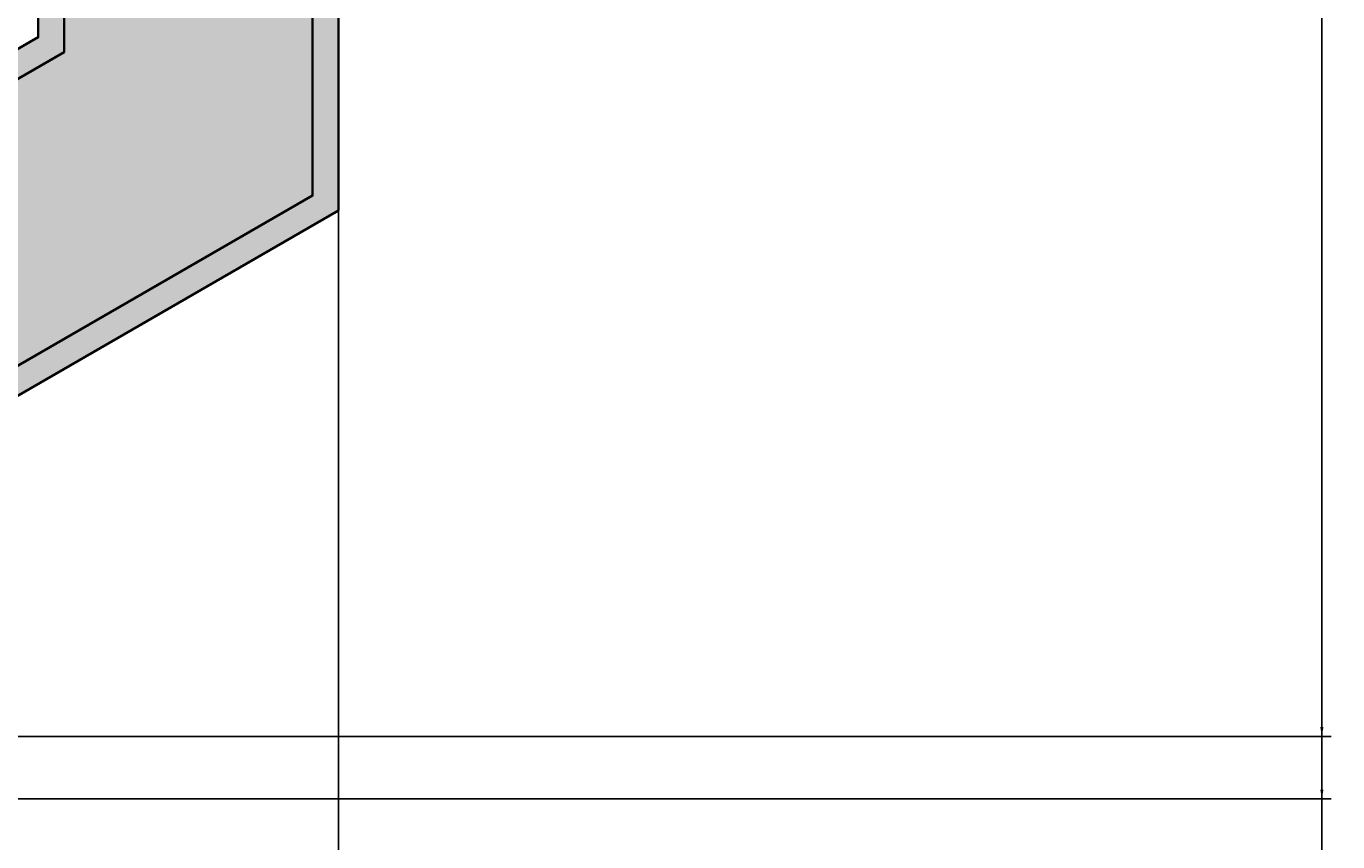
# Model space of a CAD drawing. Units: inches. Extents: x -1 to 292, y -3 to 199.
# Tile 48 of 52: x 267 to 292, y 43 to 58. Entities that reach past the tile are written whole.
import ezdxf

# ---------------------------------------------------------------- set-up
doc = ezdxf.new("R2010")
doc.units = ezdxf.units.IN
doc.header["$MEASUREMENT"] = 0
for name, color, linetype, lineweight in [('M-DIMS', 2, 'Continuous', 18), ('M-EQPM', 7, 'Continuous', 35), ('M-PATT', 8, 'Continuous', 13)]:
    doc.layers.add(name, color=color, linetype=linetype, lineweight=lineweight)
doc.styles.get("Standard").update_dxf_attribs({"font": 'arial.ttf'})
doc.dimstyles.get("Standard").update_dxf_attribs({"dimtxt": 0.18, "dimasz": 0.18, "dimexe": 0.18, "dimexo": 0.0625, "dimgap": 0.09, "dimtad": 0, "dimtih": 1, "dimtoh": 1, "dimdec": 4, "dimzin": 0, "dimdsep": 46, "dimtxsty": 'Standard', "dimcen": 0.09, "dimadec": 0, "dimazin": 0, "dimtfac": 1, "dimtdec": 4, "dimtofl": 0, "dimtmove": 0, "dimatfit": 3, "dimfxl": 1, "dimtolj": 1, "dimtzin": 0, "dimarcsym": 0})

# ---------------------------------------------------------------- blocks, each defined once
blk = doc.blocks.new('*D10')
at = {"layer": 'Defpoints', "color": 0, "transparency": 16777216}
for p in [(169.176, 99.774), (169.176, 43.391), (292.04, 43.391)]:
    blk.add_point(p, dxfattribs=at)
at = {"layer": 'M-DIMS', "color": 0, "lineweight": -2, "transparency": 16777216}
for p, q in [((169.239, 99.774), (292.22, 99.774)), ((292.04, 99.594), (292.04, 71.764)), ((292.04, 43.571), (292.04, 71.4)), ((169.239, 43.391), (292.22, 43.391))]:
    blk.add_line(p, q, dxfattribs=at)
at = {"layer": 'M-DIMS', "color": 0, "transparency": 16777216}
for points in [[(292.01, 99.594), (292.07, 99.594), (292.04, 99.774)], [(292.01, 43.571), (292.07, 43.571), (292.04, 43.391)]]:
    blk.add_solid(points, dxfattribs=at)
at = {"layer": 'M-DIMS', "color": 0, "transparency": 16777216, "insert": (292.04, 71.582), "char_height": 0.18, "attachment_point": 5}
blk.add_mtext('\\A1;56.38', dxfattribs=at)
blk = doc.blocks.new('*D25')
at = {"layer": 'Defpoints', "color": 0, "transparency": 16777216}
for p in [(273.066, 88.419), (215.241, 88.13), (273.066, -2.71)]:
    blk.add_point(p, dxfattribs=at)
at = {"layer": 'M-DIMS', "color": 0, "lineweight": -2, "transparency": 16777216}
for p, q in [((273.066, 88.357), (273.066, -2.89)), ((215.241, 88.068), (215.241, -2.89)), ((215.421, -2.71), (243.76, -2.71)), ((272.886, -2.71), (244.547, -2.71))]:
    blk.add_line(p, q, dxfattribs=at)
at = {"layer": 'M-DIMS', "color": 0, "transparency": 16777216}
for points in [[(215.421, -2.68), (215.421, -2.74), (215.241, -2.71)], [(272.886, -2.68), (272.886, -2.74), (273.066, -2.71)]]:
    blk.add_solid(points, dxfattribs=at)
at = {"layer": 'M-DIMS', "color": 0, "transparency": 16777216, "insert": (244.153, -2.71), "char_height": 0.18, "attachment_point": 5}
blk.add_mtext('\\A1;57.83', dxfattribs=at)
blk = doc.blocks.new('*D29')
at = {"layer": 'Defpoints', "color": 0, "transparency": 16777216}
for p in [(243.903, 98.567), (243.903, 44.598), (292.04, 44.598)]:
    blk.add_point(p, dxfattribs=at)
at = {"layer": 'M-DIMS', "color": 0, "lineweight": -2, "transparency": 16777216}
for p, q in [((243.966, 98.567), (292.22, 98.567)), ((292.04, 98.387), (292.04, 71.764)), ((292.04, 44.778), (292.04, 71.4)), ((243.966, 44.598), (292.22, 44.598))]:
    blk.add_line(p, q, dxfattribs=at)
at = {"layer": 'M-DIMS', "color": 0, "transparency": 16777216}
for points in [[(292.01, 98.387), (292.07, 98.387), (292.04, 98.567)], [(292.01, 44.778), (292.07, 44.778), (292.04, 44.598)]]:
    blk.add_solid(points, dxfattribs=at)
at = {"layer": 'M-DIMS', "color": 0, "transparency": 16777216, "insert": (292.04, 71.582), "char_height": 0.18, "attachment_point": 5}
blk.add_mtext('\\A1;53.97', dxfattribs=at)
blk = doc.blocks.new('*D33')
at = {"layer": 'Defpoints', "color": 0, "transparency": 16777216}
for p in [(242.955, 125.727), (292.04, 125.727), (237.933, 30.73)]:
    blk.add_point(p, dxfattribs=at)
at = {"layer": 'M-DIMS', "color": 0, "lineweight": -2, "transparency": 16777216}
for p, q in [((243.018, 125.727), (292.22, 125.727)), ((292.04, 125.547), (292.04, 78.41)), ((292.04, 30.91), (292.04, 78.046)), ((237.996, 30.73), (292.22, 30.73))]:
    blk.add_line(p, q, dxfattribs=at)
at = {"layer": 'M-DIMS', "color": 0, "transparency": 16777216}
for points in [[(292.01, 125.547), (292.07, 125.547), (292.04, 125.727)], [(292.01, 30.91), (292.07, 30.91), (292.04, 30.73)]]:
    blk.add_solid(points, dxfattribs=at)
at = {"layer": 'M-DIMS', "color": 0, "transparency": 16777216, "insert": (292.04, 78.228), "char_height": 0.18, "attachment_point": 5}
blk.add_mtext('\\A1;95', dxfattribs=at)

msp = doc.modelspace()

# ---------------------------------------------------------------- hatches: boundary and pattern name
at = {"layer": 'M-PATT'}
h = msp.add_hatch(color=256, dxfattribs=at)
h.set_gradient(color1=(0, 255, 255), color2=(0, 255, 255), tint=1, name='CYLINDER')
h.paths.add_polyline_path([(256.8092, 99.5764), (256.4077, 99.3157), (253.7155, 100.87), (251.3221, 99.3157), (248.6299, 100.87), (246.2365, 99.3157), (243.5443, 100.87), (241.1509, 99.3157), (238.4587, 100.87), (236.4209, 99.5466), (236.4209, 97.1861), (234.9209, 97.1861), (234.9209, 99.9764), (233.3731, 100.87), (230.9797, 99.3157, 1.0704128)])
h.paths.add_polyline_path([(234.4549, 44.5975, 1), (253.3518, 44.5975, 1)])
h.paths.add_polyline_path([(235.4822, 48.8821), (220.034, 57.8011), (220.034, 85.363), (232.4507, 92.5318, -0.0853739), (231.0925, 96.7051), (215.7407, 87.8418), (215.7407, 55.3224), (234.4552, 44.5176, -0.0021162), (234.4549, 44.5975, -0.1182098)])
h.paths.add_polyline_path([(222.7904, 52.8755), (221.8492, 54.5058), (223.7904, 54.6075)], flags=16)
h.paths.add_polyline_path([(216.828, 66.8912), (217.7692, 68.5216), (218.828, 66.8912)], flags=16)
h.paths.add_polyline_path([(216.8084, 83.826), (217.7497, 85.4564), (218.8084, 83.826)], flags=16)
h.paths.add_polyline_path([(226.468, 92.8803), (228.3442, 93.0348), (227.6068, 91.2362)], flags=16)
h.paths.add_polyline_path([(272.5659, 88.1304), (260.2765, 95.2257), (259.0113, 93.0196), (263.0639, 91.1046), (263.4912, 92.0087), (264.5631, 90.4612), (262.6367, 90.2004), (263.0639, 91.1046), (259.0113, 93.0196), (257.8918, 91.0677), (267.7726, 85.363), (267.7726, 57.8011), (255.5043, 50.718), (257.0663, 46.085), (272.5659, 55.0337)])
h.paths.add_polyline_path([(263.6286, 51.5636), (261.7461, 51.5636), (262.6286, 53.2956)], flags=16)
h.paths.add_polyline_path([(269.8773, 65.3608), (268.8186, 66.9911), (270.8186, 66.9911)], flags=16)
h.paths.add_polyline_path([(269.8773, 80.8843), (268.8186, 82.5146), (270.8186, 82.5146)], flags=16)
h.paths.add_polyline_path([(255.5043, 50.718), (252.3244, 48.8821, -0.1182098), (253.3518, 44.5975, -0.0177685), (253.3279, 43.9266), (257.0663, 46.085)])
h.paths.add_polyline_path([(260.2765, 95.2257), (256.7809, 97.2439, -0.0959457), (255.356, 92.5318), (257.8918, 91.0677)])
h = msp.add_hatch(color=256, dxfattribs=at)
h.set_gradient(color1=(76, 38, 47), color2=(76, 38, 47), tint=1, name='CYLINDER')
h.paths.add_polyline_path([(267.2726, 58.0898), (255.3414, 51.2013), (255.5043, 50.718), (267.7726, 57.8011), (267.7726, 85.363), (257.8918, 91.0677), (257.643, 90.634), (267.2726, 85.0743)])
h.paths.add_polyline_path([(272.5659, 55.0337), (257.0663, 46.085), (257.2293, 45.6017), (273.0659, 54.745), (273.0659, 88.4191), (260.5253, 95.6595), (260.2765, 95.2257), (272.5659, 88.1304)])
h.paths.add_polyline_path([(215.2407, 55.0337), (234.4787, 43.9266, -0.0156517), (234.4552, 44.5176), (215.7407, 55.3224), (215.7407, 87.8418), (231.0925, 96.7051, -0.0104859), (231.0257, 97.2439), (215.2407, 88.1304)])
h.paths.add_polyline_path([(220.034, 57.8011), (235.4822, 48.8821, -0.0132367), (235.7207, 49.3218), (220.534, 58.0898), (220.534, 85.0743), (232.6923, 92.0939, -0.0096587), (232.4507, 92.5318), (220.034, 85.363)])

# ---------------------------------------------------------------- linework, layer by layer
at = {"layer": 'M-EQPM'}
for points in [[(253.2639, 43.3124), (273.0659, 54.745), (273.0659, 88.4191), (256.8257, 97.7954)], [(253.3279, 43.9266), (272.5659, 55.0337), (272.5659, 88.1304), (256.7809, 97.2439)], [(252.3359, 48.8887), (267.7726, 57.8011), (267.7726, 85.363), (255.356, 92.5318)], [(252.0859, 49.3218), (267.2726, 58.0898), (267.2726, 85.0743), (255.1143, 92.0939)]]:
    msp.add_lwpolyline(points, dxfattribs=at)

# ---------------------------------------------------------------- dimensions: what is measured, and where the dimension line sits
at = {"layer": 'M-DIMS'}
for base, p1, p2, override, picture, middle in [((292.0399, 125.7269), (237.9333, 30.7296), (242.9552, 125.7269), {"dimdec": 0, "dimlfac": 1, "dimrnd": 0, "dimzin": 0, "dimdsep": 46, "dimlunit": 2}, '*D33', (292.0399, 78.2282)), ((292.0399, 43.3906), (169.176, 99.7735), (169.176, 43.3906), {"dimdec": 2, "dimlfac": 1, "dimrnd": 0, "dimzin": 0, "dimdsep": 46, "dimlunit": 2}, '*D10', (292.0399, 71.5821)), ((292.0399, 44.5975), (243.9033, 98.5666), (243.9033, 44.5975), {"dimdec": 2, "dimlfac": 1, "dimrnd": 0, "dimzin": 0, "dimdsep": 46, "dimlunit": 2}, '*D29', (292.0399, 71.5821))]:
    dim = msp.add_linear_dim(base=base, p1=p1, p2=p2, angle=90, dimstyle='Standard', override=override, dxfattribs=at)
    dim.commit()
    dim.dimension.update_dxf_attribs({"geometry": picture, "text_midpoint": middle})
dim = msp.add_linear_dim(base=(273.0659, -2.7104), p1=(215.2407, 88.1304), p2=(273.0659, 88.4191), dimstyle='Standard', override={"dimdec": 2, "dimlfac": 1, "dimrnd": 0, "dimzin": 0, "dimdsep": 46, "dimlunit": 2}, dxfattribs=at)
dim.commit()
dim.dimension.update_dxf_attribs({"geometry": '*D25', "text_midpoint": (244.1533, -2.7104)})

doc.saveas('drawing.dxf')
